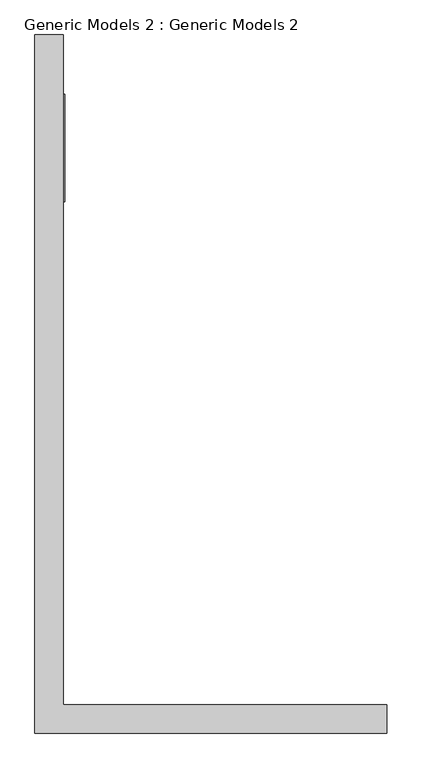
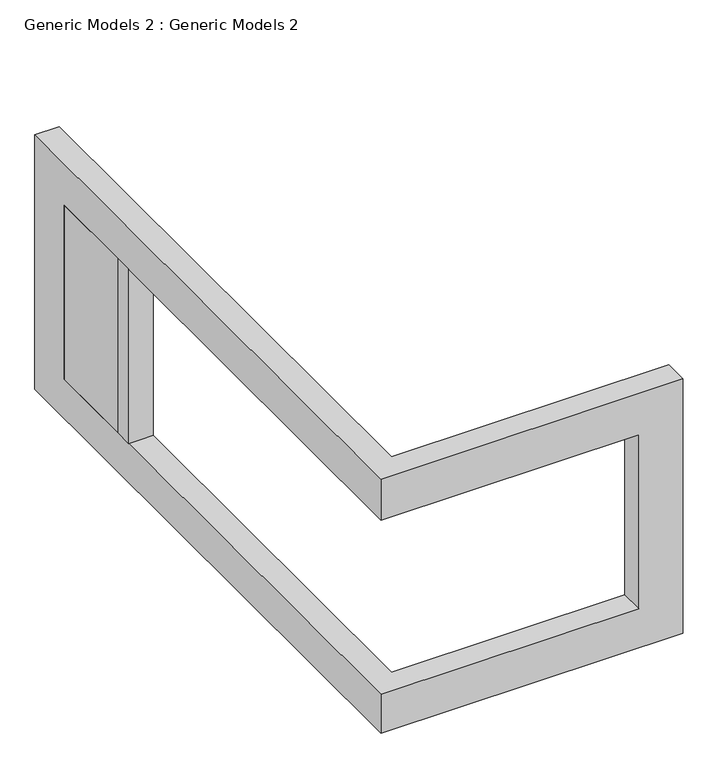
"""IFC4 building model written with IfcOpenShell, lengths in millimetres: proxy geometry, Generic Models 2 : Generic Models 2."""

from ifc_helpers import new_model, si_unit, frame, origin, place, context, project, spatial, polyline, outline, extrude, faceted_brep, source, transform, mapped, element, save


def generic_models_2_generic_models_2_8568020c(model_context):
    return source(origin(), model_context, "Body", "SolidModel", [
        extrude(outline(polyline([(-20247.4332181, -8482.0613656), (-20569.5503587, -8482.0613656), (-20569.5503587, -7326.9437275), (-20247.4332181, -7326.9437275), (-20247.4332181, -8482.0613656)])), frame((0.0, 0.0, 3560.986402), z_axis=(0.0, 0.0, 1.0), x_axis=(1.0, 0.0, 0.0)), (0.0, 0.0, 1.0), 2297.9062869),
        extrude(outline(polyline([(-20569.5503587, -8723.5026331), (-20569.5503587, -8482.0613656), (-20264.7503587, -8482.0613656), (-20264.7503587, -8723.5026331), (-20569.5503587, -8723.5026331)])), frame((0.0, 0.0, 3560.986402), z_axis=(0.0, 0.0, 1.0), x_axis=(1.0, 0.0, 0.0)), (0.0, 0.0, 1.0), 2297.9062869),
        faceted_brep([(-20264.7503587, -7326.9437275, 5858.8926889), (-20264.7503587, -7326.9437275, 3560.986402), (-20264.7503587, -13873.3526331, 3560.986402), (-20264.7503587, -13873.3526331, 3048.0), (-20264.7503587, -6691.5026331, 3048.0), (-20264.7503587, -6691.5026331, 6400.8), (-20264.7503587, -13873.3526331, 6400.8), (-20264.7503587, -13873.3526331, 5858.8926889), (-20569.5503587, -6691.5026331, 6400.8), (-20569.5503587, -6691.5026331, 3048.0), (-20569.5503587, -7326.9437275, 3560.986402), (-20569.5503587, -7326.9437275, 5858.8926889), (-20569.5503587, -14178.1526331, 5858.8926889), (-20569.5503587, -14178.1526331, 6400.8), (-20569.5503587, -14178.1526331, 3048.0), (-20569.5503587, -14178.1526331, 3560.986402), (-16797.6503587, -14178.1526331, 6400.8), (-16797.6503587, -13873.3526331, 6400.8), (-17348.2789432, -13873.3526331, 5858.8926889), (-17348.2789432, -14178.1526331, 5858.8926889), (-17348.2789432, -14178.1526331, 3560.986402), (-17348.2789432, -13873.3526331, 3560.986402), (-16797.6503587, -13873.3526331, 3048.0), (-16797.6503587, -14178.1526331, 3048.0)], [[[0, 1, 2, 3, 4, 5, 6, 7]], [[8, 5, 4, 9]], [[10, 11, 12, 13, 8, 9, 14, 15]], [[1, 0, 11, 10]], [[5, 8, 13, 16, 17, 6]], [[11, 0, 7, 18, 19, 12]], [[2, 1, 10, 15, 20, 21]], [[4, 3, 22, 23, 14, 9]], [[16, 13, 12, 19, 20, 15, 14, 23]], [[6, 17, 22, 3, 2, 21, 18, 7]], [[22, 17, 16, 23]], [[20, 19, 18, 21]]]),
    ])


if __name__ == "__main__":
    model = new_model("IFC4")
    model_context = context("Model", 3, world=origin())
    ifc_project = project(units=[si_unit("LENGTHUNIT", "METRE", prefix="MILLI")], contexts=[model_context])
    site = spatial("IfcSite", under=ifc_project)
    building = spatial("IfcBuilding", under=site)
    placement = place(None, origin())
    generic_models_2_generic_models_2_shape = generic_models_2_generic_models_2_8568020c(model_context)
    element("IfcBuildingElementProxy", 1, Name="Generic Models 2 : Generic Models 2", ObjectType="Generic Models 2 : Generic Models 2", at=placement, inside=building, context=model_context, shape_type="MappedRepresentation", body=[
        mapped(generic_models_2_generic_models_2_shape, transform((0.0, 0.0, 0.0), x_axis=(1.0, 0.0, 0.0), y_axis=(0.0, 1.0, 0.0), z_axis=(0.0, 0.0, 1.0))),
    ])
    save(model, "model.ifc")
